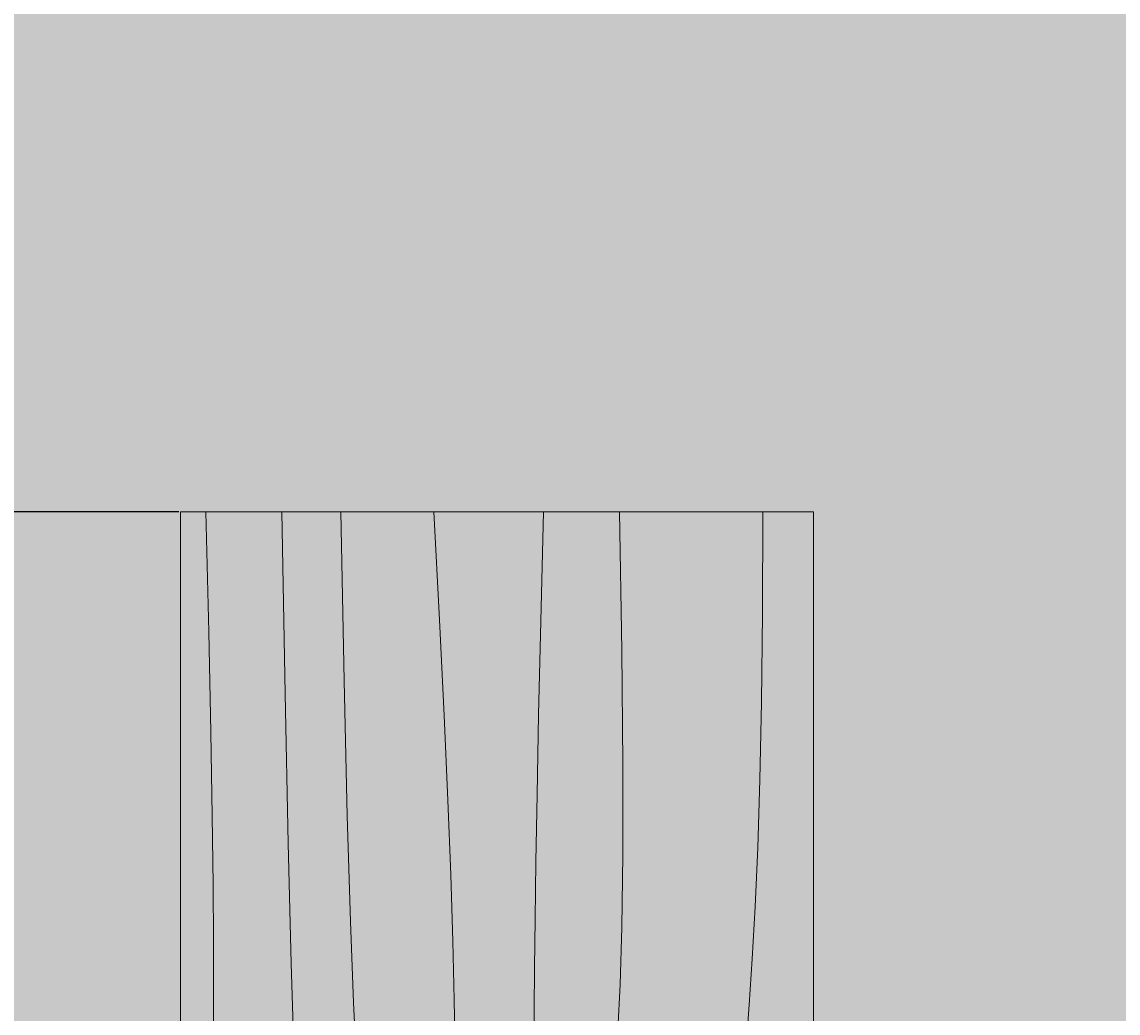
# Model space of a CAD drawing. Units: inches. Extents: x 3024 to 3952, y 1308 to 1863.
# Tile 18 of 29: x 3392 to 3430, y 1524 to 1559. Entities that reach past the tile are written whole.
import ezdxf

# ---------------------------------------------------------------- set-up
doc = ezdxf.new("R2010")
doc.units = ezdxf.units.IN
for name, color, linetype, lineweight in [('A-ANNO-DIMS', 2, 'Continuous', 18), ('A-FLOR-TILE-PATT', 7, 'Continuous', 13), ('A-FURN', 8, 'Continuous', 18), ('A-FURN-PATT', 9, 'Continuous', 13)]:
    doc.layers.add(name, color=color, linetype=linetype, lineweight=lineweight)
doc.layers.add('A-FLOR-PATT', color=254, linetype='Continuous', lineweight=13, true_color=0xfeeab9)
doc.styles.get("Standard").update_dxf_attribs({"font": 'arial.ttf'})
doc.dimstyles.get("Standard").update_dxf_attribs({"dimtxt": 0.18, "dimasz": 0.18, "dimexe": 0.18, "dimexo": 0.0625, "dimgap": 0.09, "dimtad": 0, "dimtih": 1, "dimtoh": 1, "dimdec": 4, "dimzin": 0, "dimdsep": 46, "dimtxsty": 'Standard', "dimcen": 0.09, "dimadec": 0, "dimazin": 0, "dimtfac": 1, "dimtdec": 4, "dimtofl": 0, "dimtmove": 0, "dimatfit": 3, "dimfxl": 1, "dimtolj": 1, "dimtzin": 0, "dimarcsym": 0})

# ---------------------------------------------------------------- blocks, each defined once
blk = doc.blocks.new('Table - Rectangular Woodgrain 60 x 30 in.')
for p, q in [((0, 0), (0, -30)), ((60, 0), (0, 0)), ((0, -30), (60, -30))]:
    blk.add_line(p, q)
for points in [[(0, -2.4), (4.8155, -2.418), (9.0302, -2.4688), (12.709, -2.5477), (15.9167, -2.65), (18.7181, -2.7711), (21.1781, -2.9063), (23.3616, -3.0508), (25.3333, -3.2)], [(0, -9.2), (6.5759, -9.0858), (11.9385, -9.0365), (16.2527, -9.0418), (19.6833, -9.0917), (22.3952, -9.1759), (24.5531, -9.2844)], [(0, -12.8), (5.1847, -12.9322), (9.6213, -13.0323), (13.3963, -13.1059), (16.5958, -13.1583), (19.3063, -13.1952), (21.614, -13.2219), (23.6054, -13.2439), (25.3666, -13.2667)], [(0, -18), (5.124, -17.7273), (9.6609, -17.5057), (13.6705, -17.3303), (17.2125, -17.1958), (20.3467, -17.0973), (23.1328, -17.0297), (25.6307, -16.9878)], [(0, -22.4), (8.0098, -22.2501), (14.4094, -22.1011), (19.4168, -21.9535), (23.25, -21.8083), (26.1269, -21.6663)], [(0, -25.2), (8.6355, -25.0504), (15.7026, -24.9031), (21.4049, -24.7606), (25.9458, -24.625)], [(0, -28.8), (5.6867, -28.6681), (10.45, -28.5698), (14.407, -28.5012), (17.675, -28.4584), (20.3711, -28.4374), (22.6125, -28.4344), (24.5164, -28.4455)]]:
    blk.add_lwpolyline(points)
blk = doc.blocks.new('*D32')
at = {"layer": 'A-ANNO-DIMS', "color": 0, "lineweight": -2, "transparency": 16777216}
for p, q in [((3397.088, 1541.715), (3390.23, 1541.715)), ((3390.41, 1541.535), (3390.41, 1519.428)), ((3390.41, 1496.958), (3390.41, 1519.065)), ((3397.088, 1496.778), (3390.23, 1496.778))]:
    blk.add_line(p, q, dxfattribs=at)
at = {"layer": 'A-ANNO-DIMS', "color": 0, "transparency": 16777216}
for points in [[(3390.38, 1541.535), (3390.44, 1541.535), (3390.41, 1541.715)], [(3390.38, 1496.958), (3390.44, 1496.958), (3390.41, 1496.778)]]:
    blk.add_solid(points, dxfattribs=at)
at = {"layer": 'Defpoints', "color": 0, "transparency": 16777216}
for p in [(3397.15, 1541.715), (3390.41, 1496.778), (3397.15, 1496.778)]:
    blk.add_point(p, dxfattribs=at)
at = {"layer": 'A-ANNO-DIMS', "color": 0, "transparency": 16777216, "insert": (3390.41, 1519.246), "char_height": 0.18, "attachment_point": 5}
blk.add_mtext('\\A1;TABLE 45', dxfattribs=at)

msp = doc.modelspace()

# ---------------------------------------------------------------- hatches: boundary and pattern name
at = {"layer": 'A-FLOR-PATT', "transparency": 33554528}
h = msp.add_hatch(color=256, dxfattribs=at)
h.dxf.hatch_style = 1
h.paths.add_polyline_path([(3460.764, 1688.6064), (3412.764, 1688.6064), (3412.764, 1694.6064), (3460.764, 1694.6064), (3460.764, 1778.6064), (3406.764, 1778.6064), (3406.764, 1759.9514), (3318.2981, 1759.9514), (3318.2981, 1658.6064), (3322.5356, 1658.6064), (3322.5356, 1652.6064), (3292.764, 1652.6064), (3292.764, 1778.6064), (3106.764, 1778.6064), (3106.764, 1628.6064), (3172.764, 1628.6064), (3172.764, 1532.6064), (3166.764, 1532.6064), (3166.764, 1628.6064), (3106.764, 1628.6064), (3106.764, 1356.8452), (3202.812, 1356.8452), (3202.812, 1354.2534), (3202.812, 1353.8388), (3202.812, 1351.1212), (3202.812, 1347.8452), (3277.764, 1347.8452), (3277.764, 1353.8452), (3277.764, 1356.8452), (3277.764, 1442.6064), (3460.764, 1442.6064)])
h.paths.add_polyline_path([(3216.238, 1527.2064), (3216.238, 1491.2064), (3214.663, 1491.2064), (3214.663, 1491.2409, -0.3966224), (3180.243, 1526.6064), (3163.0285, 1526.6064), (3163.0285, 1531.1064), (3161.716, 1531.1064), (3161.716, 1561.1064), (3163.0285, 1561.1064), (3163.0285, 1531.1064), (3163.0285, 1526.6064), (3180.243, 1526.6064, 0.3966224), (3214.663, 1491.2409), (3214.663, 1527.2064)], flags=16)
h.paths.add_polyline_path([(3227.364, 1649.8972), (3191.364, 1649.8972), (3191.364, 1651.4722), (3227.364, 1651.4722)], flags=16)
h.paths.add_polyline_path([(3323.1172, 1606.7362), (3323.8545, 1606.8514), (3323.8545, 1594.8241), (3323.1172, 1594.9393)], flags=16)
h.paths.add_polyline_path([(3324.2232, 1606.909), (3330.1216, 1607.8307), (3330.1216, 1614.1093), (3339.3495, 1614.1093), (3340.2711, 1620.0078), (3352.4136, 1620.0078), (3353.3353, 1614.1093), (3359.9941, 1614.1093), (3360.9157, 1620.0078), (3373.0582, 1620.0078), (3373.9799, 1614.1093), (3383.2077, 1614.1093), (3383.2077, 1607.8307), (3389.1062, 1606.909), (3389.1062, 1594.7665), (3383.2077, 1593.8449), (3383.2077, 1587.5663), (3373.9799, 1587.5663), (3373.0583, 1581.6678), (3360.9157, 1581.6678), (3359.9941, 1587.5663), (3353.3353, 1587.5663), (3352.4136, 1581.6678), (3340.2711, 1581.6678), (3339.3495, 1587.5663), (3330.1216, 1587.5663), (3330.1216, 1593.8449), (3324.2232, 1594.7665)], flags=16)
h.paths.add_polyline_path([(3236.1584, 1693.1064), (3236.1584, 1723.1064), (3237.4709, 1723.1064), (3237.4709, 1693.1064)], flags=16)
h.paths.add_polyline_path([(3373.2158, 1600.6847), (3373.7965, 1600.7303), (3374.3268, 1600.7874), (3374.8132, 1600.8531), (3375.2621, 1600.9247), (3375.6801, 1600.9991), (3376.0736, 1601.0735), (3376.6855, 1601.19), (3377.366, 1601.3023), (3378.0667, 1601.3814), (3378.8026, 1601.4123), (3379.5865, 1601.3839), (3380.4537, 1601.2948), (3381.301, 1601.1717), (3382.0317, 1601.0433), (3382.4398, 1600.9607), (3382.6252, 1600.9201), (3382.919, 1600.8507), (3382.9044, 1600.8531), (3382.842, 1600.8678), (3382.7541, 1600.8896), (3382.6252, 1600.9201), (3382.4398, 1600.9607), (3382.1868, 1601.0119), (3381.8738, 1601.0711), (3381.5125, 1601.1346), (3381.1149, 1601.1988), (3380.6928, 1601.2601), (3380.2581, 1601.3149), (3379.8226, 1601.3597), (3379.3984, 1601.3908), (3378.9944, 1601.4054), (3378.6092, 1601.4042), (3378.2384, 1601.3886), (3377.8777, 1601.36), (3377.5227, 1601.32), (3377.1691, 1601.2698), (3376.8127, 1601.211), (3376.4491, 1601.145), (3376.0736, 1601.0735), (3375.4177, 1600.9494), (3374.5542, 1600.8119), (3373.5044, 1600.6988)], flags=0)
h.paths.add_polyline_path([(3380.0253, 1596.7351), (3380.499, 1596.6659), (3380.9706, 1596.6119), (3381.4375, 1596.5791), (3381.8971, 1596.5736), (3382.5886, 1596.6167), (3382.7848, 1596.6692), (3382.1465, 1596.5706), (3381.236, 1596.5815), (3380.3199, 1596.6865)], flags=0)
h.paths.add_polyline_path([(3369.6414, 1603.9617), (3370.1589, 1604.0021), (3370.6218, 1604.0539), (3371.0335, 1604.1173), (3371.3978, 1604.1921), (3371.7181, 1604.2785), (3371.9984, 1604.3761), (3372.2441, 1604.483), (3372.4611, 1604.5972), (3372.655, 1604.7163), (3372.8317, 1604.8384), (3372.9968, 1604.9611), (3373.3703, 1605.2455), (3373.8426, 1605.5328), (3374.4624, 1605.7539), (3375.1058, 1605.8302), (3375.7221, 1605.8261), (3376.4109, 1605.76), (3377.1534, 1605.6376), (3377.8945, 1605.473), (3378.1382, 1605.409), (3377.7394, 1605.5074), (3377.3509, 1605.5937), (3376.9704, 1605.6677), (3376.5999, 1605.7288), (3376.2417, 1605.7762), (3375.8979, 1605.8092), (3375.5707, 1605.8271), (3375.2621, 1605.8291), (3374.9745, 1605.8146), (3374.7092, 1605.7832), (3374.4647, 1605.7359), (3374.239, 1605.6742), (3374.0298, 1605.5996), (3373.835, 1605.5134), (3373.6525, 1605.4171), (3373.4801, 1605.3123), (3373.3156, 1605.2002), (3373.1562, 1605.0825), (3372.7603, 1604.781), (3372.236, 1604.4588), (3371.5738, 1604.2283), (3370.8493, 1604.0794), (3369.9262, 1603.976)], flags=0)
h.paths.add_polyline_path([(3366.7533, 1606.5832), (3367.1713, 1606.5519), (3367.5378, 1606.5374), (3367.8568, 1606.5394), (3368.1325, 1606.5573), (3368.3694, 1606.5903), (3368.5717, 1606.6377), (3368.7438, 1606.6988), (3368.89, 1606.7728), (3369.0146, 1606.8591), (3369.121, 1606.9568), (3369.2094, 1607.0646), (3369.2792, 1607.181), (3369.3295, 1607.3046), (3369.3596, 1607.4339), (3369.3688, 1607.5676), (3369.3565, 1607.7042), (3369.3218, 1607.8422), (3369.2649, 1607.9804), (3369.1893, 1608.1187), (3369.0993, 1608.2569), (3368.9992, 1608.3952), (3368.8934, 1608.5334), (3368.7861, 1608.6717), (3368.6817, 1608.8099), (3368.4212, 1609.1804), (3368.2685, 1609.7106), (3368.4883, 1610.1814), (3369.0537, 1610.4604), (3369.6717, 1610.5097), (3370.2812, 1610.3612), (3370.4805, 1610.2968), (3370.1882, 1610.3839), (3369.9284, 1610.4472), (3369.6905, 1610.4842), (3369.4662, 1610.4933), (3369.2555, 1610.4765), (3369.0608, 1610.4367), (3368.884, 1610.3767), (3368.7274, 1610.2994), (3368.5931, 1610.2077), (3368.4833, 1610.1045), (3368.4002, 1609.9927), (3368.3451, 1609.8747), (3368.3166, 1609.7517), (3368.3127, 1609.6244), (3368.331, 1609.4935), (3368.3696, 1609.3597), (3368.4261, 1609.2237), (3368.4985, 1609.0863), (3368.5845, 1608.9482), (3368.6817, 1608.8099), (3368.7861, 1608.6717), (3368.8934, 1608.5334), (3368.9992, 1608.3952), (3369.0993, 1608.2569), (3369.3398, 1607.8876), (3369.3941, 1607.2896), (3368.9774, 1606.7817), (3368.3928, 1606.5742), (3367.7162, 1606.5303), (3367.0044, 1606.5585)], flags=0)
h.paths.add_polyline_path([(3362.1859, 1610.2589), (3362.5478, 1610.2845), (3362.8348, 1610.3275), (3363.0585, 1610.3863), (3363.2303, 1610.4595), (3363.3619, 1610.5457), (3363.463, 1610.6432), (3363.5376, 1610.7502), (3363.5876, 1610.8643), (3363.6153, 1610.9834), (3363.6229, 1611.1055), (3363.6125, 1611.2283), (3363.5861, 1611.3496), (3363.5462, 1611.4673), (3363.4949, 1611.5797), (3363.4358, 1611.6871), (3363.3723, 1611.7902), (3363.3081, 1611.8897), (3363.2468, 1611.9863), (3363.192, 1612.0808), (3363.0258, 1612.4261), (3363.3371, 1612.8672), (3363.9008, 1612.9782), (3364.4822, 1612.9641), (3365.1098, 1612.9074), (3365.328, 1612.8805), (3364.9615, 1612.9208), (3364.6426, 1612.9496), (3364.3668, 1612.9669), (3364.1299, 1612.9726), (3363.9276, 1612.9669), (3363.7555, 1612.9496), (3363.6093, 1612.9208), (3363.4848, 1612.8805), (3363.3782, 1612.8289), (3363.2889, 1612.7672), (3363.2169, 1612.6969), (3363.1622, 1612.6193), (3363.1247, 1612.5361), (3363.1046, 1612.4484), (3363.1017, 1612.358), (3363.1161, 1612.266), (3363.1472, 1612.1738), (3363.192, 1612.0808), (3363.2468, 1611.9863), (3363.3081, 1611.8897), (3363.3723, 1611.7902), (3363.4358, 1611.6871), (3363.6363, 1611.323), (3363.5979, 1610.7003), (3363.0863, 1610.3651), (3362.3983, 1610.2622)], flags=0)
h.paths.add_polyline_path([(3352.356, 1581.2991), (3352.2408, 1580.5618), (3340.4439, 1580.5618), (3340.3287, 1581.2991)], flags=16)
h.paths.add_polyline_path([(3340.4439, 1621.1137), (3352.2408, 1621.1137), (3352.356, 1620.3764), (3340.3287, 1620.3764)], flags=16)
h.paths.add_polyline_path([(3278.4282, 1504.7424), (3290.3831, 1504.7424), (3290.3831, 1502.7499), (3291.0473, 1502.7499), (3291.0473, 1494.7799), (3290.3831, 1494.7799), (3290.3831, 1494.1158), (3291.0473, 1494.1158), (3291.0473, 1486.1458), (3290.3831, 1486.1458), (3290.3831, 1484.1533), (3291.0473, 1484.1533), (3291.0473, 1483.4892, -0.0909091), (3291.0473, 1468.8776), (3291.0473, 1468.2135), (3290.3831, 1468.2135), (3290.3831, 1464.8926), (3278.4282, 1464.8926), (3278.4282, 1472.8626), (3277.764, 1473.5268), (3277.764, 1478.84), (3278.4282, 1479.5042)], flags=16)
h.paths.add_polyline_path([(3278.7603, 1504.4103), (3290.051, 1504.4103), (3290.051, 1465.2247), (3278.7603, 1465.2247)], flags=0)
h.paths.add_polyline_path([(3123.904, 1600.7821), (3117.9039, 1602.7821), (3117.9039, 1599.7821), (3119.4039, 1599.7821), (3119.4039, 1596.7821), (3118.4039, 1596.7821), (3118.4039, 1598.7821), (3117.9039, 1598.7821), (3117.9039, 1596.2821), (3109.9039, 1596.2821), (3109.9039, 1617.2821), (3117.9039, 1617.2821), (3117.9039, 1610.7821), (3123.9038, 1612.7821, -0.7025712), (3137.9039, 1606.7822, -0.7025621)], flags=16)
h.paths.add_polyline_path([(3123.9039, 1602.7822), (3123.9039, 1610.7822, -0.7345333), (3136.9039, 1606.7822, -0.7345297)], flags=0)
h.paths.add_polyline_path([(3177.972, 1689.6473), (3109.2405, 1689.6473), (3109.2405, 1741.1959), (3177.972, 1741.1959)], flags=16)
h.paths.add_polyline_path([(3373.0006, 1581.2991), (3372.8854, 1580.5618), (3361.0885, 1580.5618), (3360.9733, 1581.2991)], flags=16)
h.paths.add_polyline_path([(3361.0885, 1621.1137), (3372.8854, 1621.1137), (3373.0006, 1620.3764), (3360.9733, 1620.3764)], flags=16)
h.paths.add_polyline_path([(3116.9039, 1598.2821, -0.4142136), (3116.1539, 1597.2821), (3111.9039, 1597.2821, -0.4142136), (3110.9039, 1598.0321), (3110.9039, 1615.2821, -0.4142136), (3111.6539, 1616.2821), (3115.9039, 1616.2821, -0.4142136), (3116.9039, 1615.5321)], flags=0)
h.paths.add_polyline_path([(3121.6122, 1728.1369), (3121.6122, 1696.5205), (3110.2715, 1696.5205), (3110.2715, 1714.3906), (3121.6122, 1714.3906), (3121.6122, 1716.4526), (3110.2715, 1716.4526), (3110.2715, 1734.3228), (3123.3304, 1734.3228), (3123.3304, 1729.8552), (3134.6711, 1741.1959), (3134.6711, 1728.1369)], flags=0)
h.paths.add_polyline_path([(3389.4748, 1606.8514), (3390.2122, 1606.7362), (3390.2122, 1594.9393), (3389.4748, 1594.8241)], flags=16)
h.paths.add_polyline_path([(3257.6842, 1762.8281), (3259.6842, 1768.8281), (3256.6842, 1768.8281), (3256.6842, 1767.3281), (3253.6842, 1767.3281), (3253.6842, 1768.3281), (3255.6842, 1768.3281), (3255.6842, 1768.8281), (3253.1842, 1768.8281), (3253.1842, 1776.8281), (3274.1842, 1776.8281), (3274.1842, 1768.8281), (3267.6842, 1768.8281), (3269.6842, 1762.8282, -0.7025712), (3263.6843, 1748.8282, -0.7025621)], flags=16)
h.paths.add_polyline_path([(3259.6842, 1762.8281), (3267.6843, 1762.8281, -0.7345333), (3263.6842, 1749.8282, -0.7345297)], flags=0)
h.paths.add_polyline_path([(3411.264, 1715.6064), (3411.264, 1716.9189), (3441.264, 1716.9189), (3441.264, 1715.6064)], flags=16)
h.paths.add_polyline_path([(3178.3806, 1449.1876), (3178.3806, 1397.639), (3109.6491, 1397.639), (3109.6491, 1449.1876)], flags=16)
h.paths.add_polyline_path([(3397.1501, 1541.7146), (3419.6183, 1541.7146), (3419.6183, 1496.7783), (3397.1501, 1496.7783)], flags=16)
h.paths.add_polyline_path([(3254.1842, 1770.5781), (3254.1842, 1774.8281, -0.4142136), (3254.9342, 1775.8281), (3272.1842, 1775.8281, -0.4142136), (3273.1842, 1775.0781), (3273.1842, 1770.8281, -0.4142136), (3272.4342, 1769.8281), (3255.1842, 1769.8281, -0.4142136)], flags=0)
h.paths.add_polyline_path([(3403.672, 1500.7601), (3403.6016, 1500.3997), (3403.5328, 1500.0441), (3403.4662, 1499.6867), (3403.4027, 1499.3226), (3403.3464, 1498.9532), (3403.3025, 1498.5811), (3403.2759, 1498.2091), (3403.2714, 1497.8401), (3403.3064, 1497.2813), (3403.3491, 1497.1219), (3403.2689, 1497.6395), (3403.2778, 1498.3719), (3403.3635, 1499.0984), (3403.4889, 1499.8168), (3403.6016, 1500.3997), (3403.672, 1500.7601), (3403.744, 1501.1315), (3403.817, 1501.5205), (3403.891, 1501.9336), (3403.9656, 1502.3769), (3404.0404, 1502.8572), (3404.115, 1503.3786), (3404.2264, 1504.2311), (3404.2571, 1504.5223), (3404.1552, 1503.6598), (3404.0063, 1502.6193), (3403.8604, 1501.7518), (3403.744, 1501.1315)], flags=0)
h.paths.add_polyline_path([(3406.5868, 1505.0416), (3406.6121, 1504.5236), (3406.6492, 1504.0526), (3406.6956, 1503.624), (3406.7491, 1503.2333), (3406.8072, 1502.8759), (3406.8676, 1502.5473), (3406.9281, 1502.243), (3407.0268, 1501.7597), (3407.1416, 1501.1368), (3407.2087, 1500.3904), (3407.1804, 1499.6703), (3407.1078, 1498.9956), (3407.0074, 1498.3199), (3406.8809, 1497.6059), (3406.7403, 1496.9627), (3406.7418, 1496.9824), (3406.7491, 1497.0249), (3406.8229, 1497.3409), (3406.8364, 1497.4025), (3406.878, 1497.6078), (3406.9261, 1497.8614), (3406.9777, 1498.1526), (3407.0298, 1498.4712), (3407.0797, 1498.8068), (3407.1243, 1499.149), (3407.1607, 1499.4874), (3407.1859, 1499.8115), (3407.1978, 1500.1137), (3407.1969, 1500.3962), (3407.1841, 1500.6642), (3407.1609, 1500.9225), (3407.1284, 1501.1761), (3407.0876, 1501.43), (3407.0398, 1501.6891), (3406.9862, 1501.9585), (3406.8832, 1502.4628), (3406.7712, 1503.0713), (3406.6657, 1503.8424), (3406.5924, 1504.7735)], flags=0)
h.paths.add_polyline_path([(3409.2517, 1507.8962), (3409.2752, 1507.4282), (3409.3079, 1507.0076), (3409.3501, 1506.6314), (3409.4015, 1506.2969), (3409.4624, 1506.0009), (3409.5326, 1505.7406), (3409.6119, 1505.5128), (3409.6988, 1505.3131), (3409.7915, 1505.1368), (3409.8883, 1504.9792), (3409.9875, 1504.8356), (3410.0872, 1504.7015), (3410.1859, 1504.572), (3410.4508, 1504.2132), (3410.7205, 1503.6035), (3410.8059, 1502.8824), (3410.7619, 1502.0875), (3410.6122, 1501.2299), (3410.4402, 1500.6169), (3410.2538, 1500.0031), (3410.0536, 1499.3219), (3409.9909, 1499.0812), (3410.1761, 1499.7472), (3410.3596, 1500.3513), (3410.4512, 1500.6561), (3410.5312, 1500.9412), (3410.6013, 1501.226), (3410.6614, 1501.512), (3410.7111, 1501.7964), (3410.7496, 1502.0763), (3410.7764, 1502.3489), (3410.7909, 1502.6114), (3410.7926, 1502.8608), (3410.7808, 1503.0944), (3410.7553, 1503.31), (3410.7169, 1503.5087), (3410.6667, 1503.6921), (3410.6061, 1503.8621), (3410.5361, 1504.0203), (3410.4578, 1504.1686), (3410.3726, 1504.3088), (3410.2815, 1504.4424), (3410.1859, 1504.572), (3410.0872, 1504.7015), (3409.859, 1505.0083), (3409.5943, 1505.5117), (3409.4266, 1506.1336), (3409.324, 1506.8011), (3409.2586, 1507.6407)], flags=0)
h.paths.add_polyline_path([(3411.4914, 1510.5878), (3411.4432, 1510.1586), (3411.4054, 1509.775), (3411.38, 1509.4354), (3411.3681, 1509.1376), (3411.3698, 1508.8784), (3411.3843, 1508.6542), (3411.4112, 1508.4618), (3411.4497, 1508.2974), (3411.4994, 1508.1575), (3411.5595, 1508.0388), (3411.6296, 1507.9375), (3411.7097, 1507.851), (3411.802, 1507.7792), (3411.9096, 1507.7225), (3412.0353, 1507.6817), (3412.1821, 1507.6572), (3412.3528, 1507.6496), (3412.5505, 1507.6597), (3412.778, 1507.6879), (3413.0364, 1507.7341), (3413.3194, 1507.7955), (3413.6188, 1507.8687), (3413.9264, 1507.95), (3414.234, 1508.036), (3414.5333, 1508.1232), (3414.8163, 1508.208), (3415.0747, 1508.287), (3415.3023, 1508.3569), (3415.5007, 1508.4158), (3415.6733, 1508.4617), (3416.1158, 1508.5538), (3416.512, 1508.2591), (3416.716, 1507.6581), (3416.61, 1507.0003), (3416.3052, 1506.3411), (3415.8928, 1505.618), (3415.7339, 1505.3633), (3415.9914, 1505.791), (3416.201, 1506.1583), (3416.3666, 1506.4739), (3416.4925, 1506.7462), (3416.5828, 1506.9838), (3416.6413, 1507.1949), (3416.6725, 1507.3883), (3416.6799, 1507.5705), (3416.6662, 1507.7417), (3416.6339, 1507.9), (3416.5851, 1508.0436), (3416.5223, 1508.1709), (3416.4478, 1508.28), (3416.3639, 1508.3692), (3416.273, 1508.4368), (3416.1765, 1508.4815), (3416.0718, 1508.5047), (3415.9553, 1508.5079), (3415.8237, 1508.493), (3415.6733, 1508.4617), (3415.5007, 1508.4158), (3415.3327, 1508.3659), (3414.6495, 1508.157), (3414.0606, 1507.9855), (3413.4456, 1507.8229), (3412.8838, 1507.701), (3412.5505, 1507.6597), (3412.0748, 1507.6354), (3411.595, 1507.8883), (3411.398, 1508.4429), (3411.3624, 1508.9927), (3411.3854, 1509.5711), (3411.4578, 1510.3071)], flags=0)
h.paths.add_polyline_path([(3135.0797, 1449.1876), (3135.0797, 1436.1286), (3122.0208, 1436.1286), (3122.0208, 1404.5122), (3110.6801, 1404.5122), (3110.6801, 1422.3823), (3122.0208, 1422.3823), (3122.0208, 1424.4443), (3110.6801, 1424.4443), (3110.6801, 1442.3145), (3123.739, 1442.3145), (3123.739, 1437.8469)], flags=0)
h.paths.add_polyline_path([(3416.4944, 1514.2949), (3416.4837, 1513.8511), (3416.4893, 1513.4867), (3416.5102, 1513.1926), (3416.5451, 1512.9593), (3416.5929, 1512.7775), (3416.6524, 1512.6379), (3416.7224, 1512.531), (3416.8017, 1512.4488), (3416.8886, 1512.3882), (3416.9813, 1512.3476), (3417.0781, 1512.3251), (3417.1773, 1512.3189), (3417.277, 1512.3274), (3417.3757, 1512.3488), (3417.4713, 1512.3813), (3417.5627, 1512.4229), (3417.65, 1512.471), (3417.7338, 1512.5225), (3417.8146, 1512.5747), (3417.8931, 1512.6245), (3417.9699, 1512.6691), (3418.2968, 1512.8265), (3418.6505, 1512.4645), (3418.7037, 1511.9342), (3418.6693, 1511.3839), (3418.6076, 1510.8228), (3418.5777, 1510.5927), (3418.6197, 1510.9333), (3418.6525, 1511.2311), (3418.6759, 1511.4903), (3418.6899, 1511.7144), (3418.6946, 1511.9069), (3418.6899, 1512.0713), (3418.6759, 1512.2112), (3418.6525, 1512.33), (3418.6197, 1512.4311), (3418.5778, 1512.5177), (3418.5276, 1512.5903), (3418.4705, 1512.6488), (3418.4075, 1512.6933), (3418.3399, 1512.7237), (3418.2686, 1512.7401), (3418.1951, 1512.7424), (3418.1204, 1512.7307), (3418.0455, 1512.7055), (3417.9792, 1512.6736), (3417.65, 1512.471), (3417.5627, 1512.4229), (3417.4713, 1512.3813), (3417.3757, 1512.3488), (3417.277, 1512.3274), (3416.878, 1512.2936), (3416.5757, 1512.7549), (3416.492, 1513.3145), (3416.4808, 1514.0384)], flags=0)
h.paths.add_polyline_path([(3392.8223, 1481.9454), (3396.7707, 1481.9454), (3396.7707, 1480.9201), (3428.3585, 1480.9201), (3428.3585, 1481.9454), (3432.3069, 1481.9454), (3432.3069, 1464.8354, -0.266667), (3392.8223, 1464.8354)], flags=16)
h.paths.add_polyline_path([(3431.203, 1547.5428), (3450.8613, 1547.5428, -0.1904762), (3450.8614, 1484.031), (3431.203, 1484.031), (3431.203, 1488.5675), (3432.3809, 1488.5675), (3432.3809, 1543.0062), (3431.203, 1543.0062)], flags=16)
h.paths.add_polyline_path([(3451.9233, 1524.86, -0.0496282), (3451.9233, 1506.7138), (3446.7921, 1506.7138), (3446.7921, 1524.86)], flags=0)
h.paths.add_polyline_path([(3460.764, 1436.6064), (3277.764, 1436.6064), (3277.764, 1356.8452), (3277.764, 1353.8452), (3460.764, 1353.8452)], flags=17)
h.paths.add_polyline_path([(3121.3033, 1577.378), (3153.693, 1577.378), (3153.693, 1586.6752), (3121.3033, 1586.6752)], flags=24)
h.paths.add_polyline_path([(3164.1457, 1464.1276), (3210.4801, 1464.1276), (3210.4801, 1473.4247), (3164.1457, 1473.4247)], flags=24)
h.paths.add_polyline_path([(3343.1909, 1505.8863), (3373.7236, 1505.8863), (3373.7236, 1515.1773), (3343.1909, 1515.1773)], flags=24)
h.paths.add_polyline_path([(3337.6353, 1564.2926), (3370.0189, 1564.2926), (3370.0189, 1573.5836), (3337.6353, 1573.5836)], flags=24)
h.paths.add_polyline_path([(3419.204, 1753.8578), (3453.3997, 1753.8578), (3453.3997, 1762.9956), (3419.204, 1762.9956)], flags=24)
h.paths.add_polyline_path([(3341.2523, 1701.0246), (3381.0761, 1701.0246), (3381.0761, 1710.3156), (3341.2523, 1710.3156)], flags=24)
h.paths.add_polyline_path([(3245.8895, 1726.2997), (3278.2793, 1726.2997), (3278.2793, 1735.5968), (3245.8895, 1735.5968)], flags=24)
h.paths.add_polyline_path([(3128.8045, 1668.6736), (3175.1389, 1668.6736), (3175.1389, 1677.9707), (3128.8045, 1677.9707)], flags=24)
h.paths.add_polyline_path([(3345.9997, 1396.0062), (3389.09, 1396.0062), (3389.09, 1405.3033), (3345.9997, 1405.3033)], flags=24)
at = {"layer": 'A-FLOR-TILE-PATT', "transparency": 33554569}
h = msp.add_hatch(dxfattribs=at)
h.set_pattern_fill('ANGLE', color=256, scale=2)
h.set_pattern_definition([(0, (0, 0), (0, 13.97), [10.16, -3.81]), (90, (0, 0), (-13.97, 9e-16), [10.16, -3.81])])
h.paths.add_polyline_path([(3292.764, 1778.6064), (3232.764, 1778.6064), (3232.764, 1694.6064), (3236.1584, 1694.6064), (3236.1584, 1723.1064), (3237.4709, 1723.1064), (3237.4709, 1723.0777, -0.3870039), (3266.1209, 1694.6064), (3292.764, 1694.6064)])
h.paths.add_polyline_path([(3263.6843, 1748.8282, -0.7025621), (3257.6842, 1762.8281), (3259.6842, 1768.8281), (3256.6842, 1768.8281), (3256.6842, 1767.3281), (3253.6842, 1767.3281), (3253.6842, 1768.3281), (3255.6842, 1768.3281), (3255.6842, 1768.8281), (3253.1842, 1768.8281), (3253.1842, 1776.8281), (3274.1842, 1776.8281), (3274.1842, 1768.8281), (3267.6842, 1768.8281), (3269.6842, 1762.8282, -0.7025712)], flags=16)
h.paths.add_polyline_path([(3263.6842, 1749.8282, -0.7345297), (3259.6842, 1762.8281), (3267.6843, 1762.8281, -0.7345333)], flags=0)
h.paths.add_polyline_path([(3255.1842, 1769.8281, -0.4142136), (3254.1842, 1770.5781), (3254.1842, 1774.8281, -0.4142136), (3254.9342, 1775.8281), (3272.1842, 1775.8281, -0.4142136), (3273.1842, 1775.0781), (3273.1842, 1770.8281, -0.4142136), (3272.4342, 1769.8281)], flags=0)
h.paths.add_polyline_path([(3460.764, 1436.6064), (3277.764, 1436.6064), (3277.764, 1356.8452), (3277.764, 1353.8452), (3460.764, 1353.8452)])
h.paths.add_polyline_path([(3166.764, 1628.6064), (3106.764, 1628.6064), (3106.764, 1532.6064), (3133.066, 1532.6064, -0.3870039), (3161.716, 1561.0777), (3161.716, 1561.1064), (3163.0285, 1561.1064), (3163.0285, 1532.6064), (3166.764, 1532.6064)])
h.paths.add_polyline_path([(3123.904, 1600.7821), (3117.9039, 1602.7821), (3117.9039, 1599.7821), (3119.4039, 1599.7821), (3119.4039, 1596.7821), (3118.4039, 1596.7821), (3118.4039, 1598.7821), (3117.9039, 1598.7821), (3117.9039, 1596.2821), (3109.9039, 1596.2821), (3109.9039, 1617.2821), (3117.9039, 1617.2821), (3117.9039, 1610.7821), (3123.9038, 1612.7821, -0.7025712), (3137.9039, 1606.7822, -0.7025621)], flags=16)
h.paths.add_polyline_path([(3123.9039, 1602.7822), (3123.9039, 1610.7822, -0.7345333), (3136.9039, 1606.7822, -0.7345297)], flags=0)
h.paths.add_polyline_path([(3116.1539, 1597.2821), (3111.9039, 1597.2821, -0.4142136), (3110.9039, 1598.0321), (3110.9039, 1615.2821, -0.4142136), (3111.6539, 1616.2821), (3115.9039, 1616.2821, -0.4142136), (3116.9039, 1615.5321), (3116.9039, 1598.2821, -0.4142136)], flags=0)
h.paths.add_polyline_path([(3245.8895, 1726.2997), (3278.2793, 1726.2997), (3278.2793, 1735.5968), (3245.8895, 1735.5968)], flags=24)
h.paths.add_polyline_path([(3345.9997, 1396.0062), (3389.09, 1396.0062), (3389.09, 1405.3033), (3345.9997, 1405.3033)], flags=24)
h.paths.add_polyline_path([(3121.3033, 1577.378), (3153.693, 1577.378), (3153.693, 1586.6752), (3121.3033, 1586.6752)], flags=24)
at = {"layer": 'A-FURN-PATT', "transparency": 33554600}
h = msp.add_hatch(color=256, dxfattribs=at)
h.dxf.hatch_style = 1
h.paths.add_polyline_path([(3417.3334, 1524.2182), (3417.4417, 1525.8535), (3417.5429, 1527.6959), (3417.6336, 1529.794), (3417.7102, 1532.1964), (3417.7693, 1534.9516), (3417.8074, 1538.1081), (3417.8209, 1541.7146), (3412.7281, 1541.7146), (3412.8136, 1536.7897), (3412.8505, 1532.7734), (3412.8466, 1529.5424), (3412.8092, 1526.9731), (3412.7461, 1524.942), (3412.6649, 1523.3259), (3412.5731, 1522.0011), (3412.4784, 1520.8443), (3412.3871, 1519.7527), (3412.2998, 1518.707), (3412.216, 1517.7088), (3412.1351, 1516.7594), (3412.0566, 1515.8603), (3411.9799, 1515.013), (3411.9043, 1514.219), (3411.8293, 1513.4797), (3411.7548, 1512.7959), (3411.6819, 1512.1667), (3411.6125, 1511.5901), (3411.5485, 1511.0643), (3411.4914, 1510.5878), (3411.4432, 1510.1586), (3411.4054, 1509.775), (3411.38, 1509.4354), (3411.3681, 1509.1376), (3411.3698, 1508.8784), (3411.3843, 1508.6542), (3411.4112, 1508.4618), (3411.4497, 1508.2974), (3411.4994, 1508.1575), (3411.5595, 1508.0388), (3411.6296, 1507.9375), (3411.7097, 1507.851), (3411.802, 1507.7792), (3411.9096, 1507.7225), (3412.0353, 1507.6817), (3412.1821, 1507.6572), (3412.3528, 1507.6496), (3412.5505, 1507.6597), (3412.778, 1507.6879), (3413.0364, 1507.7341), (3413.3194, 1507.7955), (3413.6188, 1507.8687), (3413.9264, 1507.95), (3414.234, 1508.036), (3414.5333, 1508.1232), (3414.8163, 1508.208), (3415.0747, 1508.287), (3415.4508, 1508.4025), (3415.8572, 1508.5106), (3416.186, 1508.5015), (3416.4107, 1508.3344), (3416.5614, 1508.1136), (3416.6596, 1507.8241), (3416.6872, 1507.4795), (3416.6413, 1507.1949), (3416.5828, 1506.9838), (3416.4925, 1506.7462), (3416.3666, 1506.4739), (3416.201, 1506.1583), (3415.9914, 1505.791), (3415.7339, 1505.3633), (3415.4242, 1504.8669), (3415.0615, 1504.292), (3414.6566, 1503.6241), (3414.2236, 1502.8473), (3413.7766, 1501.946), (3413.3295, 1500.9042), (3412.8966, 1499.7062), (3412.4917, 1498.3362), (3412.1289, 1496.7783), (3417.2217, 1496.7783), (3417.334, 1498.1918), (3417.4456, 1499.5619), (3417.5561, 1500.8806), (3417.6648, 1502.1395), (3417.7712, 1503.3306), (3417.8747, 1504.4456), (3417.9746, 1505.4763), (3418.0705, 1506.4147), (3418.1617, 1507.2549), (3418.2476, 1508.0019), (3418.3277, 1508.6628), (3418.4013, 1509.245), (3418.4679, 1509.7559), (3418.5269, 1510.2027), (3418.5777, 1510.5927), (3418.6197, 1510.9333), (3418.6525, 1511.2311), (3418.6759, 1511.4903), (3418.6899, 1511.7144), (3418.6946, 1511.9069), (3418.6899, 1512.0713), (3418.6759, 1512.2112), (3418.6525, 1512.33), (3418.6197, 1512.4311), (3418.5778, 1512.5177), (3418.5276, 1512.5903), (3418.4705, 1512.6488), (3418.4075, 1512.6933), (3418.3399, 1512.7237), (3418.2686, 1512.7401), (3418.1951, 1512.7424), (3418.1204, 1512.7307), (3418.0455, 1512.7055), (3417.9699, 1512.6691), (3417.8931, 1512.6245), (3417.8146, 1512.5747), (3417.5633, 1512.4125), (3417.2709, 1512.3131), (3416.9695, 1512.3318), (3416.7549, 1512.4815), (3416.6143, 1512.696), (3416.5451, 1512.9593), (3416.5102, 1513.1926), (3416.4893, 1513.4867), (3416.4837, 1513.8511), (3416.4944, 1514.2949), (3416.5226, 1514.8277), (3416.5691, 1515.4576), (3416.6319, 1516.1871), (3416.7088, 1517.0179), (3416.7973, 1517.9515), (3416.8952, 1518.9891), (3417.0002, 1520.1323), (3417.1097, 1521.3827), (3417.2217, 1522.7416)])
h.paths.add_polyline_path([(3419.6183, 1541.7146), (3417.8209, 1541.7146), (3417.8074, 1538.1081), (3417.7693, 1534.9516), (3417.7102, 1532.1964), (3417.6336, 1529.794), (3417.5429, 1527.6959), (3417.4417, 1525.8535), (3417.3334, 1524.2182), (3417.2217, 1522.7416), (3417.1097, 1521.3827), (3417.0002, 1520.1323), (3416.8952, 1518.9891), (3416.7973, 1517.9515), (3416.7088, 1517.0179), (3416.6319, 1516.1871), (3416.5691, 1515.4576), (3416.5226, 1514.8277), (3416.4944, 1514.2949), (3416.4837, 1513.8511), (3416.4893, 1513.4867), (3416.5102, 1513.1926), (3416.5451, 1512.9593), (3416.5929, 1512.7775), (3416.6524, 1512.6379), (3416.7224, 1512.531), (3416.8017, 1512.4488), (3416.8886, 1512.3882), (3416.9813, 1512.3476), (3417.0781, 1512.3251), (3417.1773, 1512.3189), (3417.277, 1512.3274), (3417.3757, 1512.3488), (3417.4713, 1512.3813), (3417.5627, 1512.4229), (3417.65, 1512.471), (3417.7338, 1512.5225), (3417.9865, 1512.6856), (3418.237, 1512.7699), (3418.4785, 1512.6613), (3418.6304, 1512.4416), (3418.6876, 1512.1519), (3418.6969, 1511.8267), (3418.6759, 1511.4903), (3418.6525, 1511.2311), (3418.6197, 1510.9333), (3418.5777, 1510.5927), (3418.5269, 1510.2027), (3418.4679, 1509.7559), (3418.4013, 1509.245), (3418.3277, 1508.6628), (3418.2476, 1508.0019), (3418.1617, 1507.2549), (3418.0705, 1506.4147), (3417.9746, 1505.4763), (3417.8747, 1504.4456), (3417.7712, 1503.3306), (3417.6648, 1502.1395), (3417.5561, 1500.8806), (3417.4456, 1499.5619), (3417.334, 1498.1918), (3417.2217, 1496.7783), (3419.6183, 1496.7783)])
h.paths.add_polyline_path([(3412.5731, 1522.0011), (3412.6649, 1523.3259), (3412.7461, 1524.942), (3412.8092, 1526.9731), (3412.8466, 1529.5424), (3412.8505, 1532.7734), (3412.8136, 1536.7897), (3412.7281, 1541.7146), (3410.0319, 1541.7146), (3409.9329, 1537.8316), (3409.8579, 1534.5089), (3409.8028, 1531.6816), (3409.7635, 1529.2854), (3409.7359, 1527.2554), (3409.7159, 1525.5271), (3409.6994, 1524.0356), (3409.6824, 1522.7166), (3409.6614, 1521.5137), (3409.6364, 1520.405), (3409.6078, 1519.3771), (3409.5763, 1518.4164), (3409.5425, 1517.5096), (3409.5069, 1516.6432), (3409.4701, 1515.8036), (3409.4327, 1514.9775), (3409.3955, 1514.1549), (3409.3594, 1513.3392), (3409.3256, 1512.5376), (3409.2955, 1511.7571), (3409.2699, 1511.0046), (3409.2501, 1510.2873), (3409.2375, 1509.6121), (3409.233, 1508.986), (3409.2377, 1508.4145), (3409.2517, 1507.8962), (3409.2752, 1507.4282), (3409.3079, 1507.0076), (3409.3501, 1506.6314), (3409.4015, 1506.2969), (3409.4624, 1506.0009), (3409.5326, 1505.7406), (3409.6119, 1505.5128), (3409.6988, 1505.3131), (3409.7915, 1505.1368), (3409.8883, 1504.9792), (3409.9875, 1504.8356), (3410.0872, 1504.7015), (3410.3178, 1504.3987), (3410.5042, 1504.0923), (3410.643, 1503.7787), (3410.7431, 1503.4127), (3410.7808, 1503.0944), (3410.7926, 1502.8608), (3410.7909, 1502.6114), (3410.7764, 1502.3489), (3410.7496, 1502.0763), (3410.7111, 1501.7964), (3410.6614, 1501.512), (3410.6013, 1501.226), (3410.5312, 1500.9412), (3410.4512, 1500.6561), (3410.3596, 1500.3513), (3410.2538, 1500.0031), (3410.1317, 1499.5877), (3409.9909, 1499.0812), (3409.8291, 1498.4601), (3409.6438, 1497.7003), (3409.4327, 1496.7783), (3412.1289, 1496.7783), (3412.4917, 1498.3362), (3412.8966, 1499.7062), (3413.3295, 1500.9042), (3413.7766, 1501.946), (3414.2236, 1502.8473), (3414.6566, 1503.6241), (3415.0615, 1504.292), (3415.4242, 1504.8669), (3415.7339, 1505.3633), (3415.9914, 1505.791), (3416.201, 1506.1583), (3416.3666, 1506.4739), (3416.4925, 1506.7462), (3416.5828, 1506.9838), (3416.6413, 1507.1949), (3416.6725, 1507.3883), (3416.6799, 1507.5705), (3416.6662, 1507.7417), (3416.6339, 1507.9), (3416.5851, 1508.0436), (3416.5223, 1508.1709), (3416.4478, 1508.28), (3416.3639, 1508.3692), (3416.273, 1508.4368), (3416.1765, 1508.4815), (3416.0718, 1508.5047), (3415.9553, 1508.5079), (3415.8237, 1508.493), (3415.6733, 1508.4617), (3415.5007, 1508.4158), (3415.3023, 1508.3569), (3414.8599, 1508.2211), (3414.5333, 1508.1232), (3414.234, 1508.036), (3413.9264, 1507.95), (3413.6188, 1507.8687), (3413.3194, 1507.7955), (3412.8838, 1507.701), (3412.4382, 1507.6458), (3412.0995, 1507.6608), (3411.8501, 1507.7418), (3411.666, 1507.885), (3411.5226, 1508.092), (3411.4241, 1508.3695), (3411.3843, 1508.6542), (3411.3698, 1508.8784), (3411.3681, 1509.1376), (3411.38, 1509.4354), (3411.4054, 1509.775), (3411.4432, 1510.1586), (3411.4914, 1510.5878), (3411.5485, 1511.0643), (3411.6125, 1511.5901), (3411.6819, 1512.1667), (3411.7548, 1512.7959), (3411.8293, 1513.4797), (3411.9043, 1514.219), (3411.9799, 1515.013), (3412.0566, 1515.8603), (3412.1351, 1516.7594), (3412.216, 1517.7088), (3412.2998, 1518.707), (3412.3871, 1519.7527), (3412.4784, 1520.8443)])
h.paths.add_polyline_path([(3409.6614, 1521.5137), (3409.6824, 1522.7166), (3409.6994, 1524.0356), (3409.7159, 1525.5271), (3409.7359, 1527.2554), (3409.7635, 1529.2854), (3409.8028, 1531.6816), (3409.8579, 1534.5089), (3409.9329, 1537.8316), (3410.0319, 1541.7146), (3406.1374, 1541.7146), (3406.3416, 1537.8771), (3406.5076, 1534.4792), (3406.639, 1531.4763), (3406.7397, 1528.8235), (3406.8135, 1526.4762), (3406.8641, 1524.3896), (3406.8955, 1522.5188), (3406.9113, 1520.8193), (3406.915, 1519.2519), (3406.9086, 1517.8009), (3406.8933, 1516.4564), (3406.8708, 1515.2084), (3406.8423, 1514.0471), (3406.8095, 1512.9624), (3406.7738, 1511.9444), (3406.7366, 1510.9832), (3406.6994, 1510.0706), (3406.664, 1509.2052), (3406.6321, 1508.3879), (3406.6055, 1507.6192), (3406.5859, 1506.8996), (3406.5751, 1506.2298), (3406.5748, 1505.6103), (3406.5868, 1505.0416), (3406.6121, 1504.5236), (3406.6492, 1504.0526), (3406.6956, 1503.624), (3406.7491, 1503.2333), (3406.8072, 1502.8759), (3406.8676, 1502.5473), (3406.9281, 1502.243), (3407.0268, 1501.7597), (3407.1147, 1501.2828), (3407.1609, 1500.9225), (3407.1841, 1500.6642), (3407.1969, 1500.3962), (3407.1978, 1500.1137), (3407.1859, 1499.8115), (3407.1607, 1499.4874), (3407.1243, 1499.149), (3407.0797, 1498.8068), (3407.0298, 1498.4712), (3406.9777, 1498.1526), (3406.9261, 1497.8614), (3406.8567, 1497.4956), (3406.7944, 1497.2102), (3406.7609, 1497.0755), (3406.7491, 1497.0249), (3406.7418, 1496.9824), (3406.7381, 1496.9355), (3406.7367, 1496.8717), (3406.7366, 1496.7783), (3409.4327, 1496.7783), (3409.6438, 1497.7003), (3409.8291, 1498.4601), (3409.9909, 1499.0812), (3410.1317, 1499.5877), (3410.2538, 1500.0031), (3410.3596, 1500.3513), (3410.4512, 1500.6561), (3410.5312, 1500.9412), (3410.6013, 1501.226), (3410.6614, 1501.512), (3410.7111, 1501.7964), (3410.7496, 1502.0763), (3410.7764, 1502.3489), (3410.7909, 1502.6114), (3410.7926, 1502.8608), (3410.7808, 1503.0944), (3410.7553, 1503.31), (3410.7169, 1503.5087), (3410.6667, 1503.6921), (3410.6061, 1503.8621), (3410.5361, 1504.0203), (3410.4578, 1504.1686), (3410.3726, 1504.3088), (3410.2815, 1504.4424), (3410.1859, 1504.572), (3410.0109, 1504.8017), (3409.8298, 1505.064), (3409.6475, 1505.4106), (3409.5326, 1505.7406), (3409.4624, 1506.0009), (3409.4015, 1506.2969), (3409.3501, 1506.6314), (3409.3079, 1507.0076), (3409.2752, 1507.4282), (3409.2517, 1507.8962), (3409.2377, 1508.4145), (3409.233, 1508.986), (3409.2375, 1509.6121), (3409.2501, 1510.2873), (3409.2699, 1511.0046), (3409.2955, 1511.7571), (3409.3256, 1512.5376), (3409.3594, 1513.3392), (3409.3955, 1514.1549), (3409.4327, 1514.9775), (3409.4701, 1515.8036), (3409.5069, 1516.6432), (3409.5425, 1517.5096), (3409.5763, 1518.4164), (3409.6078, 1519.3771), (3409.6364, 1520.405)])
h.paths.add_polyline_path([(3406.9113, 1520.8193), (3406.8955, 1522.5188), (3406.8641, 1524.3896), (3406.8135, 1526.4762), (3406.7397, 1528.8235), (3406.639, 1531.4763), (3406.5076, 1534.4792), (3406.3416, 1537.8771), (3406.1374, 1541.7146), (3402.8421, 1541.7146), (3402.9543, 1535.7158), (3403.0659, 1530.9229), (3403.1765, 1527.1726), (3403.2852, 1524.3018), (3403.3916, 1522.1472), (3403.4951, 1520.5454), (3403.595, 1519.3334), (3403.6909, 1518.3478), (3403.7822, 1517.4515), (3403.8687, 1516.6123), (3403.9507, 1515.8241), (3404.0279, 1515.0805), (3404.1004, 1514.3756), (3404.1683, 1513.7032), (3404.2315, 1513.0571), (3404.29, 1512.4311), (3404.3436, 1511.8197), (3404.3914, 1511.2188), (3404.4322, 1510.6249), (3404.4648, 1510.0345), (3404.4879, 1509.4441), (3404.5007, 1508.8503), (3404.5017, 1508.2494), (3404.4897, 1507.6379), (3404.4643, 1507.0142), (3404.4265, 1506.3837), (3404.3783, 1505.7534), (3404.3212, 1505.1306), (3404.2571, 1504.5223), (3404.1879, 1503.936), (3404.115, 1503.3786), (3404.0404, 1502.8572), (3403.9656, 1502.3769), (3403.891, 1501.9336), (3403.817, 1501.5205), (3403.744, 1501.1315), (3403.672, 1500.7601), (3403.6016, 1500.3997), (3403.5328, 1500.0441), (3403.4662, 1499.6867), (3403.4027, 1499.3226), (3403.3464, 1498.9532), (3403.3025, 1498.5811), (3403.2759, 1498.2091), (3403.2714, 1497.8401), (3403.2941, 1497.4768), (3403.3491, 1497.1219), (3403.4412, 1496.7783), (3406.7346, 1496.7783), (3406.7393, 1496.9886), (3406.7787, 1497.147), (3406.8034, 1497.2517), (3406.8364, 1497.4025), (3406.878, 1497.6078), (3406.9261, 1497.8614), (3406.9777, 1498.1526), (3407.0298, 1498.4712), (3407.0797, 1498.8068), (3407.1243, 1499.149), (3407.1607, 1499.4874), (3407.1859, 1499.8115), (3407.1978, 1500.1137), (3407.1969, 1500.3962), (3407.1841, 1500.6642), (3407.1609, 1500.9225), (3407.1284, 1501.1761), (3407.0876, 1501.43), (3407.0398, 1501.6891), (3406.9862, 1501.9585), (3406.8832, 1502.4628), (3406.8072, 1502.8759), (3406.7491, 1503.2333), (3406.6956, 1503.624), (3406.6492, 1504.0526), (3406.6121, 1504.5236), (3406.5868, 1505.0416), (3406.5748, 1505.6103), (3406.5751, 1506.2298), (3406.5859, 1506.8996), (3406.6055, 1507.6192), (3406.6321, 1508.3879), (3406.664, 1509.2052), (3406.6994, 1510.0706), (3406.7366, 1510.9832), (3406.7738, 1511.9444), (3406.8095, 1512.9624), (3406.8423, 1514.0471), (3406.8708, 1515.2084), (3406.8933, 1516.4564), (3406.9086, 1517.8009), (3406.915, 1519.2519)])
h.paths.add_polyline_path([(3403.7822, 1517.4515), (3403.6909, 1518.3478), (3403.595, 1519.3334), (3403.4951, 1520.5454), (3403.3916, 1522.1472), (3403.2852, 1524.3018), (3403.1765, 1527.1726), (3403.0659, 1530.9229), (3402.9543, 1535.7158), (3402.8421, 1541.7146), (3400.7451, 1541.7146), (3400.8571, 1535.2472), (3400.9674, 1529.9544), (3401.0741, 1525.6837), (3401.1757, 1522.2828), (3401.2702, 1519.5992), (3401.3559, 1517.4806), (3401.4311, 1515.7745), (3401.494, 1514.3284), (3401.5433, 1513.0143), (3401.5798, 1511.8008), (3401.6046, 1510.6809), (3401.6188, 1509.6476), (3401.6237, 1508.6939), (3401.6203, 1507.8127), (3401.61, 1506.9971), (3401.5938, 1506.2399), (3401.5729, 1505.5342), (3401.5474, 1504.8723), (3401.518, 1504.2464), (3401.4846, 1503.6491), (3401.4478, 1503.0725), (3401.4078, 1502.509), (3401.3648, 1501.9509), (3401.3192, 1501.3905), (3401.2716, 1500.8219), (3401.2236, 1500.246), (3401.1775, 1499.6652), (3401.1351, 1499.0821), (3401.0986, 1498.4993), (3401.0699, 1497.9194), (3401.0513, 1497.3449), (3401.0446, 1496.7783), (3403.4412, 1496.7783), (3403.3491, 1497.1219), (3403.2941, 1497.4768), (3403.2714, 1497.8401), (3403.2759, 1498.2091), (3403.3025, 1498.5811), (3403.3464, 1498.9532), (3403.4027, 1499.3226), (3403.4662, 1499.6867), (3403.5328, 1500.0441), (3403.6016, 1500.3997), (3403.672, 1500.7601), (3403.744, 1501.1315), (3403.817, 1501.5205), (3403.891, 1501.9336), (3403.9656, 1502.3769), (3404.0404, 1502.8572), (3404.115, 1503.3786), (3404.1879, 1503.936), (3404.2571, 1504.5223), (3404.3212, 1505.1306), (3404.3783, 1505.7534), (3404.4265, 1506.3837), (3404.4643, 1507.0142), (3404.4897, 1507.6379), (3404.5017, 1508.2494), (3404.5007, 1508.8503), (3404.4879, 1509.4441), (3404.4648, 1510.0345), (3404.4322, 1510.6249), (3404.3914, 1511.2188), (3404.3436, 1511.8197), (3404.29, 1512.4311), (3404.2315, 1513.0571), (3404.1683, 1513.7032), (3404.1004, 1514.3756), (3404.0279, 1515.0805), (3403.9507, 1515.8241), (3403.8687, 1516.6123)])
h.paths.add_polyline_path([(3401.3559, 1517.4806), (3401.2702, 1519.5992), (3401.1757, 1522.2828), (3401.0741, 1525.6837), (3400.9674, 1529.9544), (3400.8571, 1535.2472), (3400.7451, 1541.7146), (3398.0489, 1541.7146), (3398.1477, 1537.4556), (3398.2213, 1533.8882), (3398.2727, 1530.9247), (3398.3047, 1528.4771), (3398.3204, 1526.4579), (3398.3227, 1524.7793), (3398.3144, 1523.3534), (3398.2985, 1522.0924), (3398.2775, 1520.9226), (3398.2525, 1519.825), (3398.2239, 1518.7946), (3398.1924, 1517.8266), (3398.1586, 1516.9159), (3398.1229, 1516.0576), (3398.0862, 1515.2468), (3398.0489, 1514.4783), (3398.0117, 1513.7461), (3397.9759, 1513.0393), (3397.9431, 1512.346), (3397.9147, 1511.6541), (3397.8921, 1510.9518), (3397.8768, 1510.2269), (3397.8703, 1509.4674), (3397.8741, 1508.6615), (3397.8906, 1507.7925), (3397.926, 1506.8259), (3397.9878, 1505.7222), (3398.0832, 1504.4425), (3398.2196, 1502.9474), (3398.4042, 1501.1979), (3398.6444, 1499.1546), (3398.9476, 1496.7783), (3401.0446, 1496.7783), (3401.0513, 1497.3449), (3401.0699, 1497.9194), (3401.0986, 1498.4993), (3401.1351, 1499.0821), (3401.1775, 1499.6652), (3401.2236, 1500.246), (3401.2716, 1500.8219), (3401.3192, 1501.3905), (3401.3648, 1501.9509), (3401.4078, 1502.509), (3401.4478, 1503.0725), (3401.4846, 1503.6491), (3401.518, 1504.2464), (3401.5474, 1504.8723), (3401.5729, 1505.5342), (3401.5938, 1506.2399), (3401.61, 1506.9971), (3401.6203, 1507.8127), (3401.6237, 1508.6939), (3401.6188, 1509.6476), (3401.6046, 1510.6809), (3401.5798, 1511.8008), (3401.5433, 1513.0143), (3401.494, 1514.3284), (3401.4311, 1515.7745)])
h.paths.add_polyline_path([(3398.3227, 1524.7793), (3398.3204, 1526.4579), (3398.3047, 1528.4771), (3398.2727, 1530.9247), (3398.2213, 1533.8882), (3398.1477, 1537.4556), (3398.0489, 1541.7146), (3397.1501, 1541.7146), (3397.1501, 1496.7783), (3398.9476, 1496.7783), (3398.6444, 1499.1546), (3398.4042, 1501.1979), (3398.2196, 1502.9474), (3398.0832, 1504.4425), (3397.9878, 1505.7222), (3397.926, 1506.8259), (3397.8906, 1507.7925), (3397.8741, 1508.6615), (3397.8703, 1509.4674), (3397.8768, 1510.2269), (3397.8921, 1510.9518), (3397.9147, 1511.6541), (3397.9431, 1512.346), (3397.9759, 1513.0393), (3398.0117, 1513.7461), (3398.0489, 1514.4783), (3398.0862, 1515.2468), (3398.1229, 1516.0576), (3398.1586, 1516.9159), (3398.1924, 1517.8266), (3398.2239, 1518.7946), (3398.2525, 1519.825), (3398.2775, 1520.9226), (3398.2985, 1522.0924), (3398.3144, 1523.3534)])

# ---------------------------------------------------------------- block references
at = {"layer": 'A-FURN', "xscale": 0.7489384925976489, "yscale": 0.7489384925976489, "zscale": 0.7489384925976489, "rotation": 270}
msp.add_blockref('Table - Rectangular Woodgrain 60 x 30 in.', (3419.6183, 1541.7146), dxfattribs=at)

# ---------------------------------------------------------------- dimensions: what is measured, and where the dimension line sits
at = {"layer": 'A-ANNO-DIMS'}
dim = msp.add_linear_dim(base=(3390.4097, 1496.7783), p1=(3397.1501, 1541.7146), p2=(3397.1501, 1496.7783), angle=270, text='TABLE <>', dimstyle='Standard', override={"dimdec": 0, "dimlfac": 1, "dimrnd": 0, "dimzin": 0, "dimdsep": 46, "dimlunit": 2}, dxfattribs=at)
dim.commit()
dim.dimension.update_dxf_attribs({"geometry": '*D32', "text_midpoint": (3390.4097, 1519.2465)})

doc.saveas('drawing.dxf')
